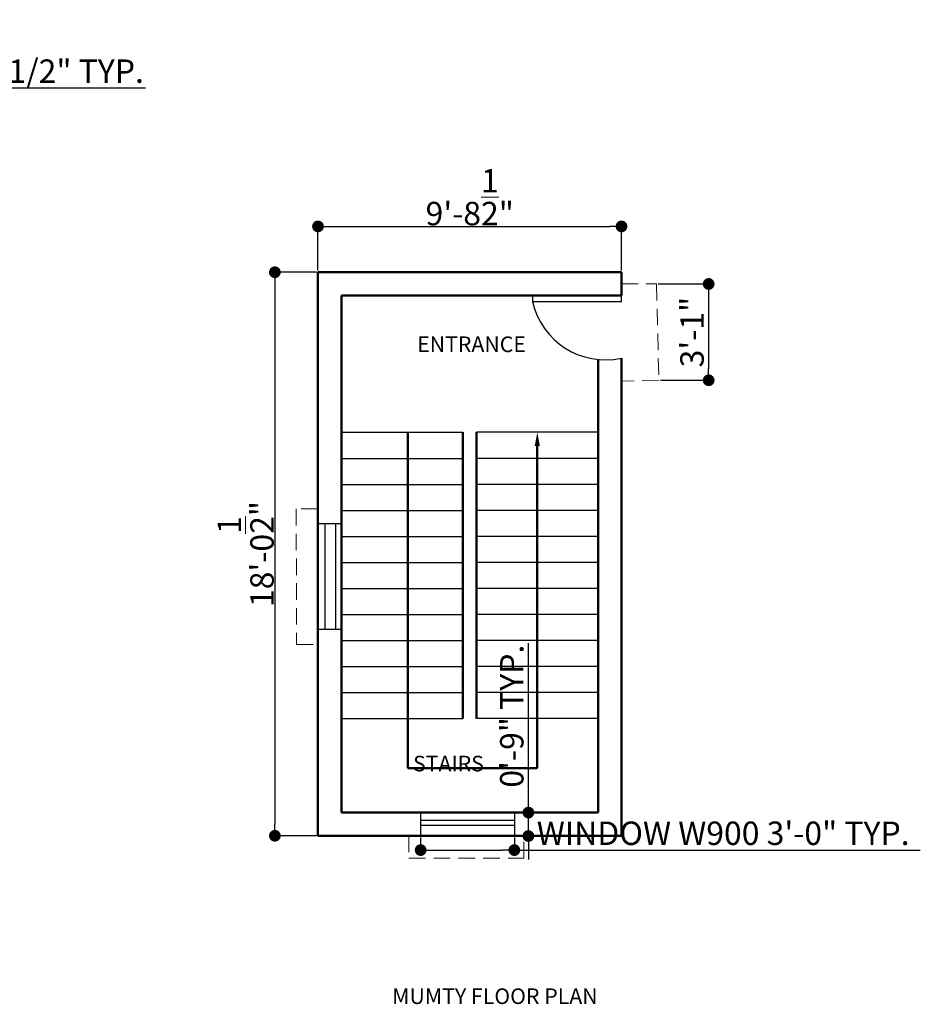
# Model space of a CAD drawing. Units: inches. Extents: x 2050 to 6806, y 2092 to 5743.
# Tile 7 of 8: x 3602 to 3948, y 2447 to 2825. Entities that reach past the tile are written whole.
import ezdxf

# ---------------------------------------------------------------- set-up
doc = ezdxf.new("R2010")
doc.units = ezdxf.units.IN
doc.linetypes.add('HIDDEN', pattern=[9.525, 6.35, -3.175])
for name, color, linetype, lineweight in [('A-ANNO-DIMS', 2, 'Continuous', 18), ('A-ANNO-TEXT', 7, 'Continuous', 25), ('A-AREA-IDEN', 7, 'Continuous', 18), ('A-DOOR', 2, 'Continuous', 25), ('A-FLOR-OVHD', 30, 'HIDDEN', 18), ('A-FLOR-STRS', 3, 'Continuous', 25), ('A-GLAZ', 6, 'Continuous', 25), ('A-WALL', 7, 'Continuous', 50)]:
    doc.layers.add(name, color=color, linetype=linetype, lineweight=lineweight)
doc.styles.get("Standard").update_dxf_attribs({"font": 'arial.ttf'})
doc.dimstyles.new('ISO-25', dxfattribs={"dimtxt": 9, "dimasz": 4.5, "dimexe": 1.25, "dimexo": 0.625, "dimtad": 1, "dimdec": 1, "dimlunit": 4, "dimtxsty": 'Standard', "dimblk": 'DOT', "dimcen": 2.5, "dimadec": 0, "dimazin": 0, "dimtfac": 1, "dimtdec": 1, "dimtmove": 0, "dimatfit": 3, "dimldrblk": 'ARCHTICK', "dimfxl": 1, "dimarcsym": 0})

# ---------------------------------------------------------------- blocks, each defined once
blk = doc.blocks.new('_Dot')
at = {"color": 0, "linetype": 'ByBlock', "lineweight": -2}
blk.add_line((-0.5, 0), (-1, 0), dxfattribs=at)
at = {"color": 0, "linetype": 'ByBlock', "const_width": 0.5}
blk.add_lwpolyline([(-0.25, 0, 1), (0.25, 0, 1)], format="xyb", close=True, dxfattribs=at)
blk = doc.blocks.new('*D44')
at = {"layer": 'A-ANNO-DIMS', "color": 0, "lineweight": -2, "transparency": 16777216}
for p, q in [((3717.01, 2728.95), (3717.01, 2747.18)), ((3833.62, 2728.95), (3833.62, 2747.18)), ((3721.51, 2745.93), (3829.12, 2745.93))]:
    blk.add_line(p, q, dxfattribs=at)
at = {"layer": 'Defpoints', "color": 0, "transparency": 16777216}
for p in [(3833.62, 2745.93), (3717.01, 2728.33), (3833.62, 2728.33)]:
    blk.add_point(p, dxfattribs=at)
at = {"layer": 'A-ANNO-DIMS', "color": 0, "lineweight": -2, "transparency": 16777216, "xscale": 4.5, "yscale": 4.5, "zscale": 4.5, "rotation": 180}
blk.add_blockref('_Dot', (3717.01, 2745.93), dxfattribs=at)
at = {"layer": 'A-ANNO-DIMS', "color": 0, "lineweight": -2, "transparency": 16777216, "xscale": 4.5, "yscale": 4.5, "zscale": 4.5}
blk.add_blockref('_Dot', (3833.62, 2745.93), dxfattribs=at)
at = {"layer": 'A-ANNO-DIMS', "color": 0, "transparency": 16777216, "insert": (3775.32, 2757.17), "char_height": 9, "attachment_point": 5}
blk.add_mtext('9\'-8{\\H1x;\\S1/2;}"', dxfattribs=at)
blk = doc.blocks.new('_ArchTick')
at = {"color": 0, "linetype": 'ByBlock', "const_width": 0.15}
blk.add_lwpolyline([(-0.5, -0.5), (0.5, 0.5)], dxfattribs=at)
blk = doc.blocks.new('*D45')
at = {"layer": 'A-ANNO-DIMS', "color": 0, "lineweight": -2, "transparency": 16777216}
for p, q in [((3847.72, 2723.83), (3868.37, 2723.83)), ((3867.12, 2719.33), (3867.12, 2691.33)), ((3848.59, 2686.83), (3868.37, 2686.83))]:
    blk.add_line(p, q, dxfattribs=at)
at = {"layer": 'Defpoints', "color": 0, "transparency": 16777216}
for p in [(3847.1, 2723.83), (3847.96, 2686.83), (3867.12, 2686.83)]:
    blk.add_point(p, dxfattribs=at)
at = {"layer": 'A-ANNO-DIMS', "color": 0, "lineweight": -2, "transparency": 16777216, "xscale": 4.5, "yscale": 4.5, "zscale": 4.5}
for p, rotation in [((3867.12, 2723.83), 90), ((3867.12, 2686.83), 270)]:
    blk.add_blockref('_Dot', p, dxfattribs=dict(at, rotation=rotation))
at = {"layer": 'A-ANNO-DIMS', "color": 0, "transparency": 16777216, "insert": (3861.9, 2705.33), "char_height": 9, "attachment_point": 5, "rotation": 90}
blk.add_mtext('3\'-1"', dxfattribs=at)
blk = doc.blocks.new('*D46')
at = {"layer": 'A-ANNO-DIMS', "color": 0, "lineweight": -2, "transparency": 16777216}
for p, q in [((3716.39, 2728.33), (3699.2, 2728.33)), ((3700.45, 2723.83), (3700.45, 2516.33)), ((3716.39, 2511.83), (3699.2, 2511.83))]:
    blk.add_line(p, q, dxfattribs=at)
at = {"layer": 'Defpoints', "color": 0, "transparency": 16777216}
for p in [(3717.01, 2728.33), (3700.45, 2511.83), (3717.01, 2511.83)]:
    blk.add_point(p, dxfattribs=at)
at = {"layer": 'A-ANNO-DIMS', "color": 0, "lineweight": -2, "transparency": 16777216, "xscale": 4.5, "yscale": 4.5, "zscale": 4.5}
for p, rotation in [((3700.45, 2728.33), 90), ((3700.45, 2511.83), 270)]:
    blk.add_blockref('_Dot', p, dxfattribs=dict(at, rotation=rotation))
at = {"layer": 'A-ANNO-DIMS', "color": 0, "transparency": 16777216, "insert": (3689.21, 2620.08), "char_height": 9, "attachment_point": 5, "rotation": 90}
blk.add_mtext('18\'-0{\\H1x;\\S1/2;}"', dxfattribs=at)
blk = doc.blocks.new('DOOR-700')
blk.add_lwpolyline([(34.15, 24.67), (0, 24.67), (0, 22.42), (34.15, 22.42)], close=True)
blk.add_arc((27.99, 28.69), 28.69, 192.6316, 282.383)
blk = doc.blocks.new('WIN-1050')
for p, q in [((0, 40.58), (9, 40.58)), ((2.5, 0), (2.5, 40.58)), ((6.5, 0), (6.5, 40.58)), ((0, 0), (9, 0))]:
    blk.add_line(p, q)
blk = doc.blocks.new('WIN-900')
for p, q in [((0, 9), (0, 0)), ((36, 9), (36, 0)), ((36, 5.99), (0, 5.99)), ((36, 3.99), (0, 3.99)), ((36, 3.99), (0, 3.99))]:
    blk.add_line(p, q)
blk = doc.blocks.new('SUNSHADE-C')
for p, q in [((0, 8.26), (0, 0)), ((52.07, 0), (52.07, 8.25)), ((0, 0), (52.07, 0))]:
    blk.add_line(p, q)
blk = doc.blocks.new('*D69')
at = {"layer": 'A-ANNO-DIMS', "color": 0, "lineweight": -2, "transparency": 16777216}
for p, q in [((3756.46, 2511.12), (3756.46, 2505.09)), ((3792.46, 2511.12), (3792.46, 2505.09)), ((3760.96, 2506.34), (3787.96, 2506.34)), ((3792.46, 2506.34), (3948.44, 2506.34))]:
    blk.add_line(p, q, dxfattribs=at)
at = {"layer": 'Defpoints', "color": 0, "transparency": 16777216}
for p in [(3756.46, 2511.74), (3792.46, 2511.74), (3792.46, 2506.34)]:
    blk.add_point(p, dxfattribs=at)
at = {"layer": 'A-ANNO-DIMS', "color": 0, "lineweight": -2, "transparency": 16777216, "xscale": 4.5, "yscale": 4.5, "zscale": 4.5, "rotation": 180}
blk.add_blockref('_Dot', (3756.46, 2506.34), dxfattribs=at)
at = {"layer": 'A-ANNO-DIMS', "color": 0, "lineweight": -2, "transparency": 16777216, "xscale": 4.5, "yscale": 4.5, "zscale": 4.5}
blk.add_blockref('_Dot', (3792.46, 2506.34), dxfattribs=at)
at = {"layer": 'A-ANNO-DIMS', "color": 0, "transparency": 16777216, "insert": (3872.7, 2511.63), "char_height": 9, "attachment_point": 5}
blk.add_mtext('WINDOW W900 3\'-0" TYP.', dxfattribs=at)
blk = doc.blocks.new('*D70')
at = {"layer": 'A-ANNO-DIMS', "color": 0, "lineweight": -2, "transparency": 16777216}
for p, q in [((3797.86, 2525.24), (3797.86, 2585.85)), ((3793.09, 2520.74), (3799.11, 2520.74)), ((3797.86, 2511.74), (3797.86, 2520.74)), ((3793.09, 2511.74), (3799.11, 2511.74)), ((3797.86, 2507.24), (3797.86, 2502.74))]:
    blk.add_line(p, q, dxfattribs=at)
at = {"layer": 'Defpoints', "color": 0, "transparency": 16777216}
for p in [(3792.46, 2520.74), (3797.86, 2520.74), (3792.46, 2511.74)]:
    blk.add_point(p, dxfattribs=at)
at = {"layer": 'A-ANNO-DIMS', "color": 0, "lineweight": -2, "transparency": 16777216, "xscale": 4.5, "yscale": 4.5, "zscale": 4.5}
for p, rotation in [((3797.86, 2520.74), 270), ((3797.86, 2511.74), 90)]:
    blk.add_blockref('_Dot', p, dxfattribs=dict(at, rotation=rotation))
at = {"layer": 'A-ANNO-DIMS', "color": 0, "transparency": 16777216, "insert": (3792.64, 2557.8), "char_height": 9, "attachment_point": 5, "rotation": 90}
blk.add_mtext('0\'-9" TYP.', dxfattribs=at)
blk = doc.blocks.new('*D80')
at = {"layer": 'A-ANNO-DIMS', "color": 0, "lineweight": -2, "transparency": 16777216}
for p, q in [((3551.67, 2806.32), (3551.67, 2797.88)), ((3562.12, 2806.32), (3562.12, 2797.88)), ((3556.17, 2799.13), (3557.62, 2799.13)), ((3562.12, 2799.13), (3650.69, 2799.13))]:
    blk.add_line(p, q, dxfattribs=at)
at = {"layer": 'Defpoints', "color": 0, "transparency": 16777216}
for p in [(3551.67, 2806.95), (3562.12, 2806.95), (3562.12, 2799.13)]:
    blk.add_point(p, dxfattribs=at)
at = {"layer": 'A-ANNO-DIMS', "color": 0, "lineweight": -2, "transparency": 16777216, "xscale": 4.5, "yscale": 4.5, "zscale": 4.5, "rotation": 180}
blk.add_blockref('_Dot', (3551.67, 2799.13), dxfattribs=at)
at = {"layer": 'A-ANNO-DIMS', "color": 0, "lineweight": -2, "transparency": 16777216, "xscale": 4.5, "yscale": 4.5, "zscale": 4.5}
blk.add_blockref('_Dot', (3562.12, 2799.13), dxfattribs=at)
at = {"layer": 'A-ANNO-DIMS', "color": 0, "transparency": 16777216, "insert": (3608.66, 2804.41), "char_height": 9, "attachment_point": 5}
blk.add_mtext('0\'-10 1/2" TYP.', dxfattribs=at)

msp = doc.modelspace()

# ---------------------------------------------------------------- linework, layer by layer
at = {"layer": 'A-FLOR-OVHD'}
for p, q in [((3833.62, 2723.83), (3847.1, 2723.83)), ((3847.1, 2723.83), (3847.96, 2686.83)), ((3847.96, 2686.83), (3833.62, 2686.54)), ((3751.96, 2511.83), (3751.96, 2503.17)), ((3796.04, 2503.17), (3796.04, 2511.83)), ((3751.96, 2503.17), (3796.04, 2503.17))]:
    msp.add_line(p, q, dxfattribs=at)
at = {"layer": 'A-FLOR-STRS'}
for p, q in [((3726.01, 2666.83), (3762.01, 2666.83)), ((3726.01, 2666.83), (3772.7, 2666.83)), ((3824.62, 2666.83), (3777.93, 2666.83)), ((3824.62, 2666.83), (3788.62, 2666.83)), ((3726.01, 2656.83), (3772.7, 2656.83)), ((3824.62, 2656.83), (3777.93, 2656.83)), ((3726.01, 2646.83), (3772.7, 2646.83)), ((3824.62, 2646.83), (3777.93, 2646.83)), ((3726.01, 2636.83), (3772.7, 2636.83)), ((3824.62, 2636.83), (3777.93, 2636.83)), ((3726.01, 2626.83), (3772.7, 2626.83)), ((3824.62, 2626.83), (3777.93, 2626.83)), ((3726.01, 2616.83), (3772.7, 2616.83)), ((3824.62, 2616.83), (3777.93, 2616.83)), ((3726.01, 2606.83), (3772.7, 2606.83)), ((3824.62, 2606.83), (3777.93, 2606.83)), ((3726.01, 2596.83), (3772.7, 2596.83)), ((3824.62, 2596.83), (3777.93, 2596.83)), ((3726.01, 2586.83), (3772.7, 2586.83)), ((3824.62, 2586.83), (3777.93, 2586.83)), ((3726.01, 2576.83), (3772.7, 2576.83)), ((3824.62, 2576.83), (3777.93, 2576.83)), ((3726.01, 2566.83), (3772.7, 2566.83)), ((3824.62, 2566.83), (3777.93, 2566.83)), ((3726.01, 2556.83), (3772.7, 2556.83)), ((3824.62, 2556.83), (3777.93, 2556.83)), ((3726.01, 2520.83), (3772.7, 2520.83))]:
    msp.add_line(p, q, dxfattribs=at)
at = {"layer": 'A-WALL'}
for p, q in [((3726.01, 2728.33), (3717.01, 2728.33)), ((3717.01, 2728.33), (3717.01, 2719.33)), ((3833.62, 2728.33), (3726.01, 2728.33)), ((3833.62, 2719.33), (3833.62, 2728.33)), ((3717.01, 2520.83), (3717.01, 2719.33)), ((3833.62, 2719.33), (3726.01, 2719.33)), ((3726.01, 2520.83), (3726.01, 2719.33)), ((3824.62, 2694.8), (3824.62, 2666.83)), ((3833.62, 2666.83), (3833.62, 2695.33)), ((3751.5, 2537.84), (3751.5, 2666.83)), ((3772.7, 2666.83), (3772.7, 2556.83)), ((3777.93, 2666.83), (3777.93, 2556.83)), ((3824.62, 2666.83), (3824.62, 2520.83)), ((3833.62, 2666.83), (3833.62, 2511.83)), ((3801.28, 2661.55), (3801.28, 2537.84)), ((3833.62, 2547.83), (3833.62, 2511.83)), ((3801.28, 2537.84), (3751.5, 2537.84)), ((3717.01, 2520.83), (3717.01, 2511.83)), ((3824.62, 2520.83), (3726.01, 2520.83)), ((3717.01, 2511.83), (3717.01, 2511.83)), ((3717.01, 2511.83), (3726.01, 2511.83)), ((3833.62, 2511.83), (3726.01, 2511.83))]:
    msp.add_line(p, q, dxfattribs=at)
msp.add_lwpolyline([(3801.28, 2666.83, 0, 2, 0), (3801.28, 2661.55, 2, 2, 0)], format="xyseb", dxfattribs=at)

# ---------------------------------------------------------------- block references
at = {"layer": 'A-DOOR'}
msp.add_blockref('DOOR-700', (3799.47, 2694.66), dxfattribs=at)
at = {"layer": 'A-FLOR-OVHD', "rotation": 270.1385157652038}
msp.add_blockref('SUNSHADE-C', (3708.65, 2637.4), dxfattribs=at)
at = {"layer": 'A-GLAZ', "rotation": 180}
msp.add_blockref('WIN-1050', (3726.18, 2631.69), dxfattribs=at)
at = {"layer": 'A-GLAZ'}
msp.add_blockref('WIN-900', (3756.46, 2511.74), dxfattribs=at)

# ---------------------------------------------------------------- texts
at = {"layer": 'A-ANNO-TEXT'}
msp.add_text('MUMTY FLOOR PLAN', height=6, dxfattribs=at).set_placement((3745.52, 2447.2))
at = {"layer": 'A-AREA-IDEN'}
for s, p in [('ENTRANCE', (3755.12, 2697.66)), ('STAIRS', (3753.53, 2536.57))]:
    msp.add_text(s, height=6, dxfattribs=at).set_placement(p)

# ---------------------------------------------------------------- dimensions: what is measured, and where the dimension line sits
at = {"layer": 'A-ANNO-DIMS'}
for base, p1, p2, text, picture, middle in [((3562.1196, 2799.133), (3551.6715, 2806.9451), (3562.1196, 2806.9451), '<> TYP.', '*D80', (3608.6562, 2804.4114)), ((3792.46, 2506.34), (3756.46, 2511.74), (3792.46, 2511.74), 'WINDOW W900 <> TYP.', '*D69', (3872.7, 2511.63))]:
    dim = msp.add_linear_dim(base=base, p1=p1, p2=p2, text=text, dimstyle='ISO-25', override={"dimdec": 1, "dimlfac": 1, "dimrnd": 0, "dimzin": 1, "dimdsep": 46, "dimlunit": 4, "dimfrac": 2}, dxfattribs=at)
    dim.commit()
    dim.dimension.update_dxf_attribs({"geometry": picture, "text_midpoint": middle})
dim = msp.add_linear_dim(base=(3833.62, 2745.93), p1=(3717.01, 2728.33), p2=(3833.62, 2728.33), dimstyle='ISO-25', override={"dimclrd": 0, "dimclre": 0, "dimclrt": 0}, dxfattribs=at)
dim.commit()
dim.dimension.update_dxf_attribs({"geometry": '*D44', "text_midpoint": (3775.32, 2757.17)})
for base, p1, p2, picture, middle in [((3700.45, 2511.83), (3717.01, 2728.33), (3717.01, 2511.83), '*D46', (3689.21, 2620.08)), ((3867.12, 2686.83), (3847.1, 2723.83), (3847.96, 2686.83), '*D45', (3861.9, 2705.33))]:
    dim = msp.add_linear_dim(base=base, p1=p1, p2=p2, angle=90, dimstyle='ISO-25', override={"dimclrd": 0, "dimclre": 0, "dimclrt": 0}, dxfattribs=at)
    dim.commit()
    dim.dimension.update_dxf_attribs({"geometry": picture, "text_midpoint": middle})
dim = msp.add_linear_dim(base=(3797.86, 2520.74), p1=(3792.46, 2511.74), p2=(3792.46, 2520.74), angle=90, text='<> TYP.', dimstyle='ISO-25', override={"dimdec": 1, "dimlfac": 1, "dimrnd": 0, "dimzin": 1, "dimdsep": 46, "dimlunit": 4, "dimfrac": 2}, dxfattribs=at)
dim.commit()
dim.dimension.update_dxf_attribs({"geometry": '*D70', "text_midpoint": (3792.64, 2557.8)})

doc.saveas('drawing.dxf')
